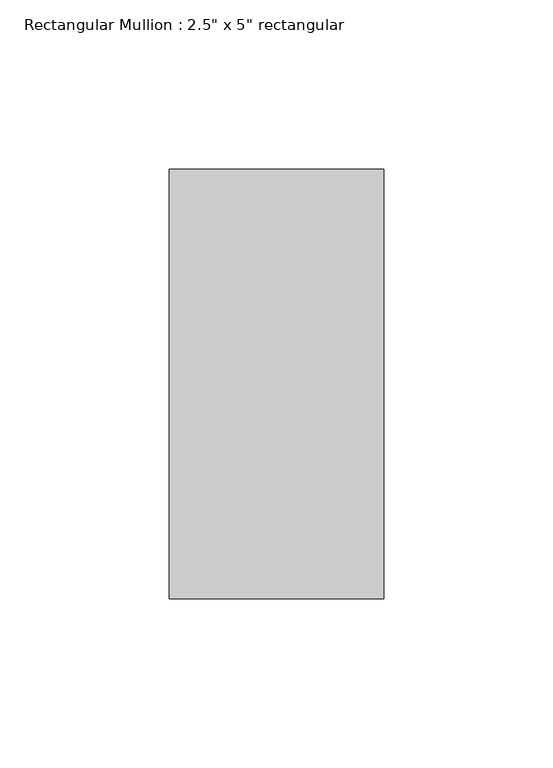
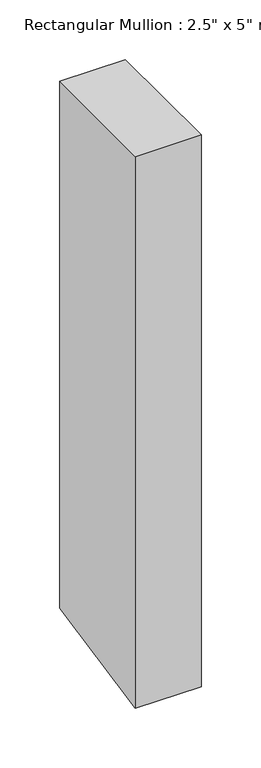
"""IFC4 building model written with IfcOpenShell, lengths in millimetres: member geometry."""

from ifc_helpers import new_model, si_unit, frame, origin, place, context, project, spatial, polyline, outline, extrude, source, transform, mapped, element, save


def member_8659189c(model_context):
    return source(origin(), model_context, "Body", "SweptSolid", [
        extrude(outline(polyline([(-63.5, 0.0), (63.5, 0.0), (63.5, -539.2536382), (-63.5, -564.5155089), (-63.5, 0.0)])), frame((-63.5, 0.0, 0.0), z_axis=(1.0, 0.0, 0.0), x_axis=(0.0, 1.0, 0.0)), (0.0, 0.0, 1.0), 63.5),
    ])


if __name__ == "__main__":
    model = new_model("IFC4")
    model_context = context("Model", 3, world=origin())
    ifc_project = project(units=[si_unit("LENGTHUNIT", "METRE", prefix="MILLI")], contexts=[model_context])
    site = spatial("IfcSite", under=ifc_project)
    building = spatial("IfcBuilding", under=site)
    placement = place(None, origin())
    member_shape = member_8659189c(model_context)
    element("IfcMember", 1, ObjectType="Rectangular Mullion : 2.5\" x 5\" rectangular", at=placement, inside=building, context=model_context, shape_type="MappedRepresentation", body=[
        mapped(member_shape, transform((0.0, 0.0, 0.0), x_axis=(1.0, 0.0, 0.0), y_axis=(0.0, 1.0, 0.0), z_axis=(0.0, 0.0, 1.0))),
    ])
    save(model, "model.ifc")

# Revit data of these elements
# Type "Rectangular Mullion : 2.5\" x 5\" rectangular"
#   built-in parameter 1007304 = 0.416667 (stored number, unit not read)
#   built-in parameter 1007301 = 0.104167 (stored number, unit not read)
#   built-in parameter 1007300 = 0.104167 (stored number, unit not read)
# Element 1 (IfcMember, "Rectangular Mullion : 2.5\" x 5\" rectangular")
#   Materials on its faces: "Iron, Ductile"
# Materials
#   "Iron, Ductile": class "Metal", colour RGB 0 0 0, transparency 0, Description = "Ductile cast iron", Cost = 0
